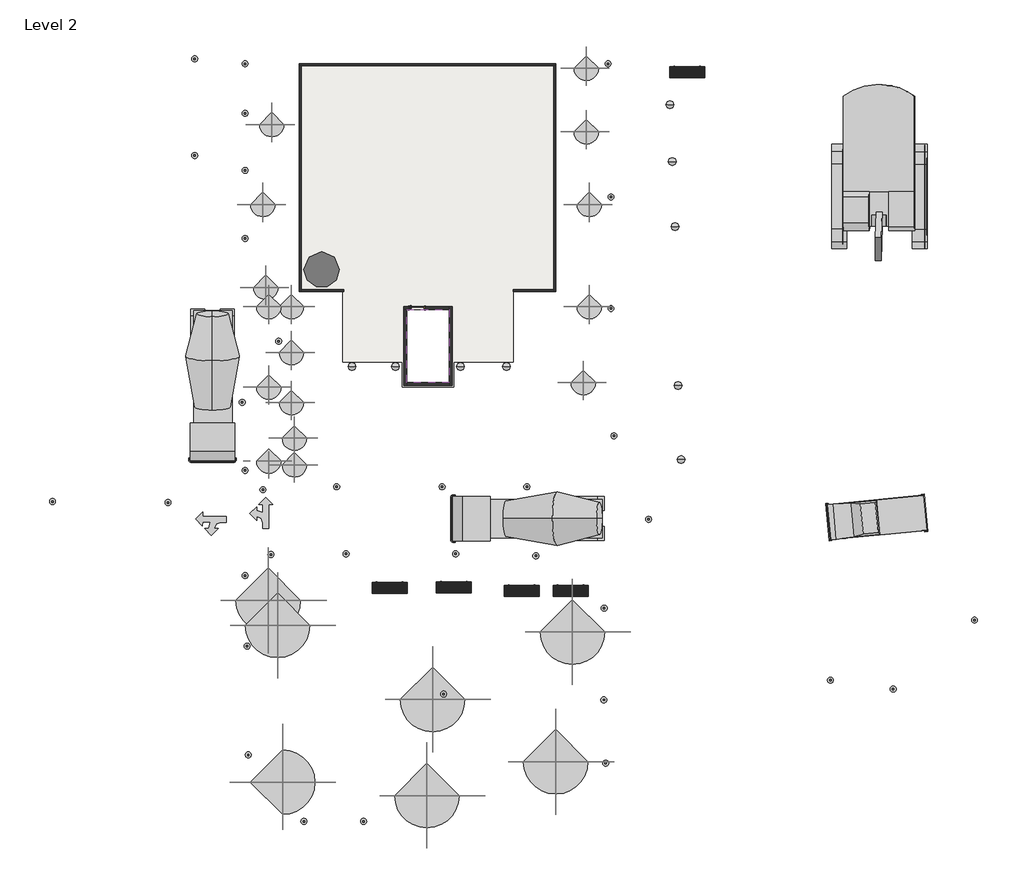
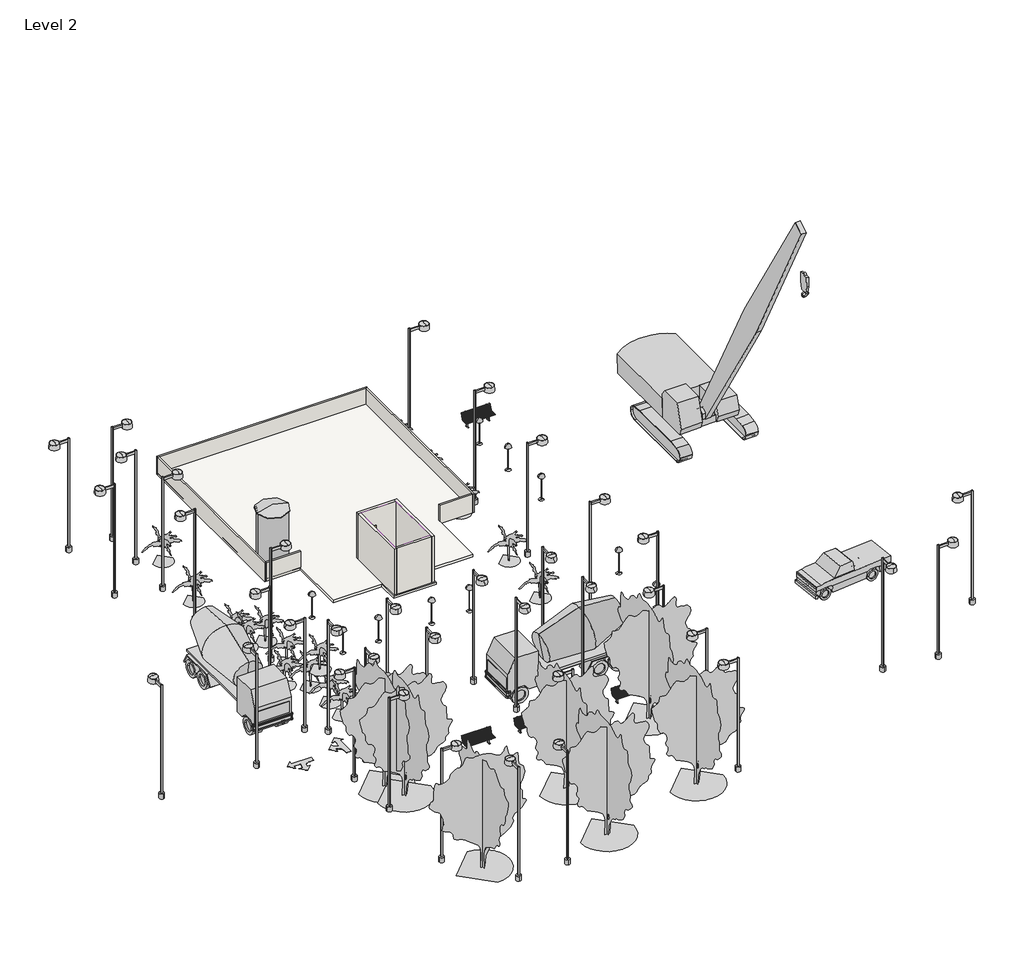
# One storey, incomplete: 46 light fixtures, 34 geographic elements, 9 walls, 1 covering, 1 door, 1 proxy, 1 slab.
# Revit data of these elements (continued)
# Elements 14, 15, 16, 17, 18, 19, 20, 21, 22, 23, 24, 25, 26, 27, 28, 29 (IfcGeographicElement, "M_RPC Tree - Tropical : Australian Tree Fern - 1.8 Meters")
#   Phase Created = New Construction
# Element 30 (IfcGeographicElement, "M_Truck - Pick-Up : Pick-Up Truck")
#   Phase Created = New Construction
#   Materials on its faces: "Metal - Paint Finish - Blue, Sky", "Steel", "Rubber - Black"
# Elements 31, 32, 33, 34, 35, 36, 37 (IfcGeographicElement, "RPC Tree - Deciduous : Honey Locust - 25'")
#   Phase Created = New Construction
# Element 38 (IfcLightFixture, "M_Floor Lamp - Hemispheric : 100W - 277V")
#   Mark = "38"
#   Phase Created = New Construction
#   Materials on its faces: "Steel, Chrome Plated", "Plastic, Lamp Shade"
# Element 39 (IfcLightFixture, "M_Floor Lamp - Hemispheric : 100W - 277V")
#   Mark = "39"
#   Phase Created = New Construction
#   Materials on its faces: "Steel, Chrome Plated", "Plastic, Lamp Shade"
# Element 40 (IfcLightFixture, "M_Floor Lamp - Hemispheric : 100W - 277V")
#   Mark = "40"
#   Phase Created = New Construction
#   Materials on its faces: "Steel, Chrome Plated", "Plastic, Lamp Shade"
# Element 41 (IfcLightFixture, "M_Floor Lamp - Hemispheric : 100W - 277V")
#   Mark = "41"
#   Phase Created = New Construction
#   Materials on its faces: "Steel, Chrome Plated", "Plastic, Lamp Shade"
# Element 42 (IfcLightFixture, "M_Floor Lamp - Hemispheric : 100W - 277V")
#   Mark = "42"
#   Phase Created = New Construction
#   Materials on its faces: "Steel, Chrome Plated", "Plastic, Lamp Shade"
# Element 43 (IfcLightFixture, "M_Floor Lamp - Hemispheric : 60W - 120V")
#   Mark = "1"
#   Phase Created = New Construction
#   Materials on its faces: "Steel, Chrome Plated", "Plastic, Lamp Shade"
# Element 44 (IfcLightFixture, "M_Floor Lamp - Hemispheric : 60W - 120V")
#   Mark = "2"
#   Phase Created = New Construction
#   Materials on its faces: "Steel, Chrome Plated", "Plastic, Lamp Shade"
# Element 45 (IfcLightFixture, "M_Floor Lamp - Hemispheric : 60W - 120V")
#   Mark = "3"
#   Phase Created = New Construction
#   Materials on its faces: "Steel, Chrome Plated", "Plastic, Lamp Shade"
# Element 46 (IfcLightFixture, "M_Floor Lamp - Hemispheric : 60W - 120V")
#   Mark = "5"
#   Phase Created = New Construction
#   Materials on its faces: "Steel, Chrome Plated", "Plastic, Lamp Shade"
# Element 47 (IfcLightFixture, "M_Floor Lamp - Hemispheric : 60W - 120V")
#   Mark = "6"
#   Phase Created = New Construction
#   Materials on its faces: "Steel, Chrome Plated", "Plastic, Lamp Shade"
# Element 48 (IfcLightFixture, "M_Street Light - Standard : 400W Halogen - 120V")
#   Mark = "7"
#   Phase Created = New Construction
#   Materials on its faces: "Steel, Paint Finish, Dark Gray, Matte", "Glass, Frosted"
# Element 49 (IfcLightFixture, "M_Street Light - Standard : 400W Halogen - 120V")
#   Mark = "8"
#   Phase Created = New Construction
#   Materials on its faces: "Steel, Paint Finish, Dark Gray, Matte", "Glass, Frosted"
# Element 50 (IfcLightFixture, "M_Street Light - Standard : 400W Halogen - 120V")
#   Mark = "9"
#   Phase Created = New Construction
#   Materials on its faces: "Steel, Paint Finish, Dark Gray, Matte", "Glass, Frosted"
# Element 51 (IfcLightFixture, "M_Street Light - Standard : 400W Halogen - 120V")
#   Mark = "10"
#   Phase Created = New Construction
#   Materials on its faces: "Steel, Paint Finish, Dark Gray, Matte", "Glass, Frosted"
# Element 52 (IfcLightFixture, "M_Street Light - Standard : 400W Halogen - 120V")
#   Mark = "11"
#   Phase Created = New Construction
#   Materials on its faces: "Steel, Paint Finish, Dark Gray, Matte", "Glass, Frosted"
# Element 53 (IfcLightFixture, "M_Street Light - Standard : 400W Halogen - 120V")
#   Mark = "12"
#   Phase Created = New Construction
#   Materials on its faces: "Steel, Paint Finish, Dark Gray, Matte", "Glass, Frosted"
# Element 54 (IfcLightFixture, "M_Street Light - Standard : 400W Halogen - 120V")
#   Mark = "13"
#   Phase Created = New Construction
#   Materials on its faces: "Steel, Paint Finish, Dark Gray, Matte", "Glass, Frosted"
# Element 55 (IfcLightFixture, "M_Street Light - Standard : 400W Halogen - 120V")
#   Mark = "14"
#   Phase Created = New Construction
#   Materials on its faces: "Steel, Paint Finish, Dark Gray, Matte", "Glass, Frosted"
# Element 56 (IfcLightFixture, "M_Street Light - Standard : 400W Halogen - 120V")
#   Mark = "15"
#   Phase Created = New Construction
#   Materials on its faces: "Steel, Paint Finish, Dark Gray, Matte", "Glass, Frosted"
# Element 57 (IfcLightFixture, "M_Street Light - Standard : 400W Halogen - 120V")
#   Mark = "16"
#   Phase Created = New Construction
#   Materials on its faces: "Steel, Paint Finish, Dark Gray, Matte", "Glass, Frosted"
# Element 58 (IfcLightFixture, "M_Street Light - Standard : 400W Halogen - 120V")
#   Mark = "17"
#   Phase Created = New Construction
#   Materials on its faces: "Steel, Paint Finish, Dark Gray, Matte", "Glass, Frosted"
# Element 59 (IfcLightFixture, "M_Street Light - Standard : 400W Halogen - 120V")
#   Mark = "18"
#   Phase Created = New Construction
#   Materials on its faces: "Steel, Paint Finish, Dark Gray, Matte", "Glass, Frosted"
# Element 60 (IfcLightFixture, "M_Street Light - Standard : 400W Halogen - 120V")
#   Mark = "19"
#   Phase Created = New Construction
#   Materials on its faces: "Steel, Paint Finish, Dark Gray, Matte", "Glass, Frosted"
# Element 61 (IfcLightFixture, "M_Street Light - Standard : 400W Halogen - 120V")
#   Mark = "20"
#   Phase Created = New Construction
#   Materials on its faces: "Steel, Paint Finish, Dark Gray, Matte", "Glass, Frosted"
# Element 62 (IfcLightFixture, "M_Street Light - Standard : 400W Halogen - 120V")
#   Mark = "21"
#   Phase Created = New Construction
#   Materials on its faces: "Steel, Paint Finish, Dark Gray, Matte", "Glass, Frosted"
# Element 63 (IfcLightFixture, "M_Street Light - Standard : 400W Halogen - 120V")
#   Mark = "24"
#   Phase Created = New Construction
#   Materials on its faces: "Steel, Paint Finish, Dark Gray, Matte", "Glass, Frosted"
# Element 64 (IfcLightFixture, "M_Street Light - Standard : 400W Halogen - 120V")
#   Mark = "25"
#   Phase Created = New Construction
#   Materials on its faces: "Steel, Paint Finish, Dark Gray, Matte", "Glass, Frosted"
# Element 65 (IfcLightFixture, "M_Street Light - Standard : 400W Halogen - 120V")
#   Mark = "26"
#   Phase Created = New Construction
#   Materials on its faces: "Steel, Paint Finish, Dark Gray, Matte", "Glass, Frosted"
# Element 66 (IfcLightFixture, "M_Street Light - Standard : 400W Halogen - 120V")
#   Mark = "27"
#   Phase Created = New Construction
#   Materials on its faces: "Steel, Paint Finish, Dark Gray, Matte", "Glass, Frosted"
# Element 67 (IfcLightFixture, "M_Street Light - Standard : 400W Halogen - 120V")
#   Mark = "28"
#   Phase Created = New Construction
#   Materials on its faces: "Steel, Paint Finish, Dark Gray, Matte", "Glass, Frosted"
# Element 68 (IfcLightFixture, "M_Street Light - Standard : 400W Halogen - 120V")
#   Mark = "29"
#   Phase Created = New Construction
#   Materials on its faces: "Steel, Paint Finish, Dark Gray, Matte", "Glass, Frosted"
# Element 69 (IfcLightFixture, "M_Street Light - Standard : 400W Halogen - 120V")
#   Mark = "30"
#   Phase Created = New Construction
#   Materials on its faces: "Steel, Paint Finish, Dark Gray, Matte", "Glass, Frosted"
# Element 70 (IfcLightFixture, "M_Street Light - Standard : 400W Halogen - 120V")
#   Mark = "31"
#   Phase Created = New Construction
#   Materials on its faces: "Steel, Paint Finish, Dark Gray, Matte", "Glass, Frosted"
# Element 71 (IfcLightFixture, "M_Street Light - Standard : 400W Halogen - 120V")
#   Mark = "32"
#   Phase Created = New Construction
#   Materials on its faces: "Steel, Paint Finish, Dark Gray, Matte", "Glass, Frosted"
# Element 72 (IfcLightFixture, "M_Street Light - Standard : 400W Halogen - 120V")
#   Mark = "33"
#   Phase Created = New Construction
#   Materials on its faces: "Steel, Paint Finish, Dark Gray, Matte", "Glass, Frosted"
# Element 73 (IfcLightFixture, "M_Street Light - Standard : 400W Halogen - 120V")
#   Mark = "34"
#   Phase Created = New Construction
#   Materials on its faces: "Steel, Paint Finish, Dark Gray, Matte", "Glass, Frosted"
# Element 74 (IfcLightFixture, "M_Street Light - Standard : 400W Halogen - 120V")
#   Mark = "35"
#   Phase Created = New Construction
#   Materials on its faces: "Steel, Paint Finish, Dark Gray, Matte", "Glass, Frosted"
# Element 75 (IfcLightFixture, "M_Street Light - Standard : 400W Halogen - 120V")
#   Mark = "36"
#   Phase Created = New Construction
#   Materials on its faces: "Steel, Paint Finish, Dark Gray, Matte", "Glass, Frosted"
# Element 76 (IfcLightFixture, "M_Street Light - Standard : 400W Halogen - 120V")
#   Mark = "37"
#   Phase Created = New Construction
#   Materials on its faces: "Steel, Paint Finish, Dark Gray, Matte", "Glass, Frosted"
# Element 77 (IfcLightFixture, "M_Street Light - Standard : 400W Halogen - 480V")
#   Mark = "44"
#   Phase Created = New Construction
#   Materials on its faces: "Steel, Paint Finish, Dark Gray, Matte", "Glass, Frosted"
# Element 78 (IfcLightFixture, "M_Street Light - Standard : 400W Halogen - 480V")
#   Mark = "46"
#   Phase Created = New Construction
#   Materials on its faces: "Steel, Paint Finish, Dark Gray, Matte", "Glass, Frosted"
# Element 79 (IfcLightFixture, "M_Street Light - Standard : 400W Halogen - 480V")
#   Mark = "47"
#   Phase Created = New Construction
#   Materials on its faces: "Steel, Paint Finish, Dark Gray, Matte", "Glass, Frosted"
# Element 80 (IfcLightFixture, "M_Street Light - Standard : 400W Halogen - 480V")
#   Mark = "48"
#   Phase Created = New Construction
#   Materials on its faces: "Steel, Paint Finish, Dark Gray, Matte", "Glass, Frosted"
# Element 81 (IfcLightFixture, "M_Street Light - Standard : 400W Halogen - 480V")
#   Mark = "49"
#   Phase Created = New Construction
#   Materials on its faces: "Steel, Paint Finish, Dark Gray, Matte", "Glass, Frosted"
# Element 82 (IfcLightFixture, "M_Street Light - Standard : 400W Halogen - 480V")
#   Mark = "50"
#   Phase Created = New Construction
#   Materials on its faces: "Steel, Paint Finish, Dark Gray, Matte", "Glass, Frosted"
# Element 83 (IfcLightFixture, "M_Street Light - Standard : 400W Halogen - 480V")
#   Mark = "51"
#   Phase Created = New Construction
#   Materials on its faces: "Steel, Paint Finish, Dark Gray, Matte", "Glass, Frosted"
# Element 84 (IfcSlab, "Generic - 6\"")
#   built-in parameter 1001955 = 3.14159 (stored number, unit not read)
#   Height Offset From Level = 0' - 6"
#   Phase Created = New Construction
#   Materials on its faces: "Default Floor", "LVW1", "Concrete Masonry Units"
# Elements 85, 86 (IfcWall, "Generic - 4\"")
#   Top Offset = 0' - 0"
#   Base Offset = 0' - 0"
#   Unconnected Height = 4' - 0"
#   wall height = 4' - 0"
#   Phase Created = New Construction
#   Base Constraint = Level 2
#   Materials on its faces: "Paint - White", "Default Wall"
# Elements 87, 88, 89 (IfcWall, "Generic - 4\"")
#   Top Offset = 0' - 0"
#   Base Offset = 0' - 0"
#   Unconnected Height = 4' - 0"
#   wall height = 4' - 0"
#   Phase Created = New Construction
#   Base Constraint = Level 2
#   Materials on its faces: "Default Wall", "Paint - White"
# Element 90 (IfcWall, "Generic - 6\"")
#   Top Offset = 0' - 0"
#   Base Offset = 0' - 0"
#   Unconnected Height = 10' - 6"
#   wall height = 10' - 6"
#   Phase Created = New Construction
#   Base Constraint = Level 2
#   Materials on its faces: "LVW1", "Default Wall"
# Elements 91, 92, 93 (IfcWall, "Generic - 6\"")
#   Top Offset = 0' - 0"
#   Base Offset = 0' - 0"
#   Unconnected Height = 10' - 6"
#   wall height = 10' - 6"
#   Phase Created = New Construction
#   Base Constraint = Level 2
#   Materials on its faces: "Default Wall", "LVW1"
# Materials
#   "Default": colour RGB 127 127 127, transparency 0, Cost = 0
#   "Acoustic Ceiling Tile 24 x 48": class "Generic", colour RGB 229 229 229, transparency 0, Description = "Acoustic Ceiling Tile 24 x 48", Cost = 0
#   "Cherry": class "Wood", colour RGB 226 177 128, transparency 0, Description = "Prunus Serotina", Cost = 0
#   "Aluminum": class "Metal", colour RGB 247 247 247, transparency 0, Description = "Aluminum 6061", Cost = 0
#   "Metal, Paint Finish, White, Matte": class "Metal", colour RGB 247 247 239, transparency 0, Description = "Paint finished steel", Cost = 0
#   "Plastic, Opaque Black": class "Plastic", colour RGB 0 0 0, transparency 0.7, Description = "Plastic, generic, opaque black", Cost = 0
#   "Wood - Teak": class "Wood", colour RGB 120 73 19, transparency 0
#   "Steel, Paint Finish, Dark Gray, Matte": class "Metal", colour RGB 98 98 98, transparency 0, Description = "Steel, paint finish, dark gray, matte", Cost = 0
#   "Rubber - Black": class "Rubber", colour RGB 0 0 0, transparency 0
#   "Metal - Paint Finish - Blue, Sky": class "Paint", colour RGB 69 113 122, transparency 0
#   "Plastic, Lamp Shade": class "Glass", colour RGB 250 244 225, transparency 0.58, Description = "physical material", Cost = 0
#   "Steel, Chrome Plated": class "Metal", colour RGB 17 17 17, transparency 0, Description = "Chromiuim plated steel", Cost = 0
#   "Glass, Frosted": class "Glass", colour RGB 250 244 225, transparency 0.55, Description = "physical material", Cost = 0
#   "Concrete Masonry Units": class "Masonry", colour RGB 227 227 227, transparency 0, Description = "Concrete masonry units", Cost = 0
#   "Paint - White": class "Paint", colour RGB 249 249 249, transparency 0
#   "Steel": class "Metal", colour RGB 128 128 128, transparency 0, Description = "Steel, mill finish", Cost = 0
#   "Default Floor": colour RGB 128 128 128, transparency 0, Cost = 0
#   "LVW1": class "Generic", colour RGB 120 120 120, transparency 0, Cost = 0
#   "Default Wall": colour RGB 128 128 128, transparency 0, Cost = 0
